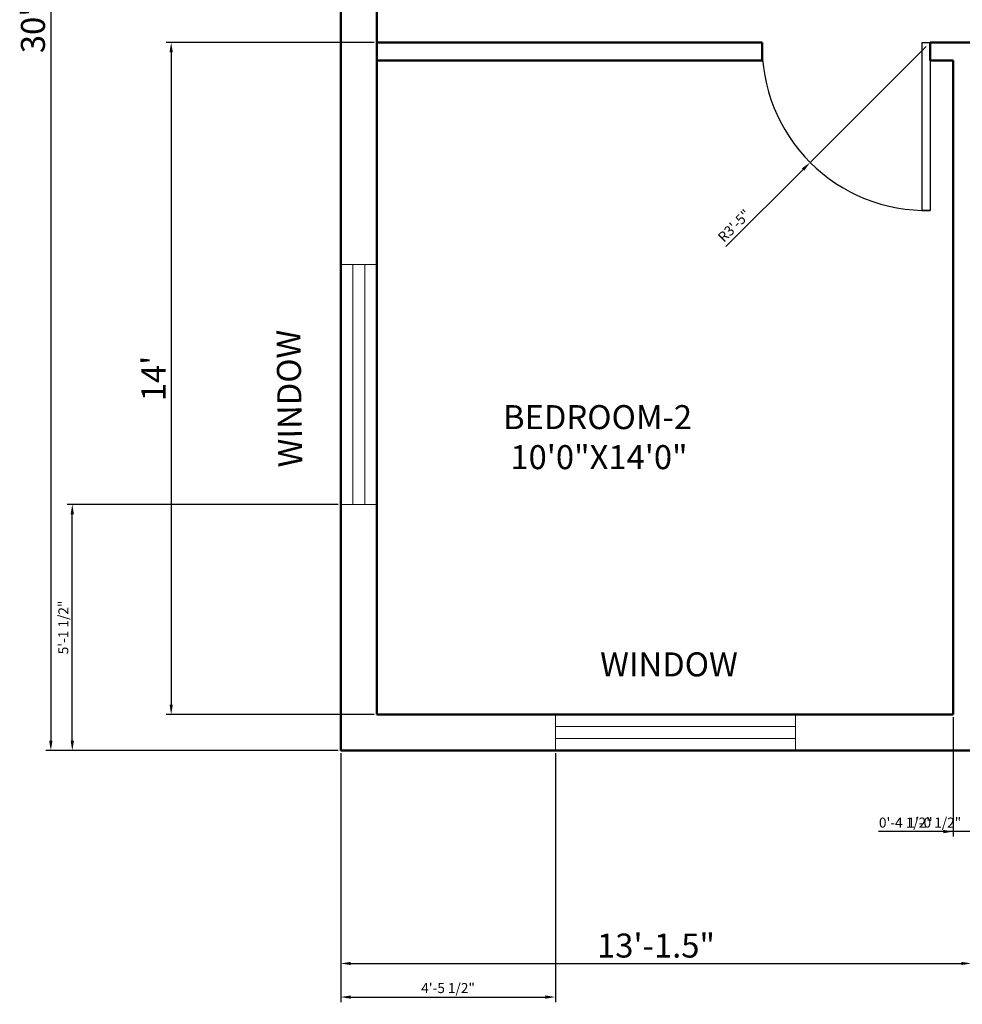
# Model space of a CAD drawing. Units: inches. Extents: x 259417 to 260009, y 246275 to 246915.
# Tile 1 of 4: x 259417 to 259653, y 246340 to 246587. Entities that reach past the tile are written whole.
import ezdxf

# ---------------------------------------------------------------- set-up
doc = ezdxf.new("R2010")
doc.units = ezdxf.units.IN
for name, color, linetype, lineweight in [('A-ANNO-DIMS', 2, 'Continuous', 18), ('A-ANNO-TEXT', 7, 'Continuous', 18), ('A-AREA-IDEN', 7, 'Continuous', 25), ('A-DOOR', 3, 'Continuous', 25), ('A-GLAZ', 4, 'Continuous', 18), ('A-WALL', 7, 'Continuous', 50)]:
    doc.layers.add(name, color=color, linetype=linetype, lineweight=lineweight)
doc.styles.get("Standard").update_dxf_attribs({"font": 'arial.ttf'})
doc.dimstyles.new('ISO-25', dxfattribs={"dimtxt": 2.5, "dimasz": 2.5, "dimexe": 1.25, "dimexo": 0.625, "dimtad": 1, "dimdec": 1, "dimlunit": 3, "dimtxsty": 'Standard', "dimcen": 2.5, "dimadec": 0, "dimazin": 0, "dimtfac": 1, "dimtdec": 1, "dimtmove": 0, "dimatfit": 3, "dimfxl": 1, "dimarcsym": 0})

# ---------------------------------------------------------------- blocks, each defined once
blk = doc.blocks.new('*D9')
at = {"layer": 'A-ANNO-DIMS', "color": 0, "lineweight": -2, "transparency": 16777216}
for p, q in [((259496.97, 246763.84), (259423.92, 246763.84)), ((259425.17, 246761.34), (259425.17, 246406.34)), ((259496.97, 246403.84), (259423.92, 246403.84))]:
    blk.add_line(p, q, dxfattribs=at)
at = {"layer": 'A-ANNO-DIMS', "color": 0, "transparency": 16777216}
for points in [[(259424.75, 246761.34), (259425.59, 246761.34), (259425.17, 246763.84)], [(259424.75, 246406.34), (259425.59, 246406.34), (259425.17, 246403.84)]]:
    blk.add_solid(points, dxfattribs=at)
at = {"layer": 'Defpoints', "color": 0, "transparency": 16777216}
for p in [(259497.59, 246763.84), (259425.17, 246403.84), (259497.59, 246403.84)]:
    blk.add_point(p, dxfattribs=at)
at = {"layer": 'A-ANNO-DIMS', "color": 0, "transparency": 16777216, "insert": (259421.48, 246583.84), "char_height": 6, "attachment_point": 5, "rotation": 90}
blk.add_mtext("30'", dxfattribs=at)
blk = doc.blocks.new('*D10')
at = {"layer": 'A-ANNO-DIMS', "color": 0, "lineweight": -2, "transparency": 16777216}
for p, q in [((259505.97, 246580.84), (259453.98, 246580.84)), ((259455.23, 246578.34), (259455.23, 246415.34)), ((259505.97, 246412.84), (259453.98, 246412.84))]:
    blk.add_line(p, q, dxfattribs=at)
at = {"layer": 'A-ANNO-DIMS', "color": 0, "transparency": 16777216}
for points in [[(259454.81, 246578.34), (259455.64, 246578.34), (259455.23, 246580.84)], [(259454.81, 246415.34), (259455.64, 246415.34), (259455.23, 246412.84)]]:
    blk.add_solid(points, dxfattribs=at)
at = {"layer": 'Defpoints', "color": 0, "transparency": 16777216}
for p in [(259506.59, 246580.84), (259455.23, 246412.84), (259506.59, 246412.84)]:
    blk.add_point(p, dxfattribs=at)
at = {"layer": 'A-ANNO-DIMS', "color": 0, "transparency": 16777216, "insert": (259451.59, 246496.84), "char_height": 6, "attachment_point": 5, "rotation": 90}
blk.add_mtext("14'", dxfattribs=at)
blk = doc.blocks.new('*D20')
at = {"layer": 'A-ANNO-DIMS', "color": 0, "lineweight": -2, "transparency": 16777216}
for p, q in [((259497.59, 246403.22), (259497.59, 246349.38)), ((259655.09, 246403.22), (259655.09, 246349.38)), ((259500.09, 246350.63), (259652.59, 246350.63))]:
    blk.add_line(p, q, dxfattribs=at)
at = {"layer": 'A-ANNO-DIMS', "color": 0, "transparency": 16777216}
for points in [[(259500.09, 246351.04), (259500.09, 246350.21), (259497.59, 246350.63)], [(259652.59, 246351.04), (259652.59, 246350.21), (259655.09, 246350.63)]]:
    blk.add_solid(points, dxfattribs=at)
at = {"layer": 'Defpoints', "color": 0, "transparency": 16777216}
for p in [(259497.59, 246403.84), (259655.09, 246403.84), (259655.09, 246350.63)]:
    blk.add_point(p, dxfattribs=at)
at = {"layer": 'A-ANNO-DIMS', "color": 0, "transparency": 16777216, "insert": (259576.34, 246354.32), "char_height": 6, "attachment_point": 5}
blk.add_mtext('13\'-1.5"', dxfattribs=at)
blk = doc.blocks.new('WIN-60x9')
for p, q in [((0, 9), (0, 0)), ((60, 9), (60, 0)), ((60, 6), (0, 6)), ((60, 3), (0, 3))]:
    blk.add_line(p, q)
blk = doc.blocks.new('*D38')
at = {"layer": 'A-ANNO-DIMS', "color": 0, "lineweight": -2, "transparency": 16777216}
for p, q in [((259496.97, 246465.37), (259429.27, 246465.37)), ((259430.52, 246406.34), (259430.52, 246462.87)), ((259496.97, 246403.84), (259429.27, 246403.84))]:
    blk.add_line(p, q, dxfattribs=at)
at = {"layer": 'A-ANNO-DIMS', "color": 0, "transparency": 16777216}
for points in [[(259430.11, 246462.87), (259430.94, 246462.87), (259430.52, 246465.37)], [(259430.11, 246406.34), (259430.94, 246406.34), (259430.52, 246403.84)]]:
    blk.add_solid(points, dxfattribs=at)
at = {"layer": 'Defpoints', "color": 0, "transparency": 16777216}
for p in [(259430.52, 246465.37), (259497.59, 246465.37), (259497.59, 246403.84)]:
    blk.add_point(p, dxfattribs=at)
at = {"layer": 'A-ANNO-DIMS', "color": 0, "transparency": 16777216, "insert": (259428.61, 246434.61), "char_height": 2.5, "attachment_point": 5, "rotation": 90}
blk.add_mtext('5\'-1 1/2"', dxfattribs=at)
blk = doc.blocks.new('*D39')
at = {"layer": 'A-ANNO-DIMS', "color": 0, "lineweight": -2, "transparency": 16777216}
for p, q in [((259497.59, 246403.22), (259497.59, 246340.98)), ((259551.19, 246403.22), (259551.19, 246340.98)), ((259500.09, 246342.23), (259548.69, 246342.23))]:
    blk.add_line(p, q, dxfattribs=at)
at = {"layer": 'A-ANNO-DIMS', "color": 0, "transparency": 16777216}
for points in [[(259500.09, 246342.64), (259500.09, 246341.81), (259497.59, 246342.23)], [(259548.69, 246342.64), (259548.69, 246341.81), (259551.19, 246342.23)]]:
    blk.add_solid(points, dxfattribs=at)
at = {"layer": 'Defpoints', "color": 0, "transparency": 16777216}
for p in [(259497.59, 246403.84), (259551.19, 246403.84), (259551.19, 246342.23)]:
    blk.add_point(p, dxfattribs=at)
at = {"layer": 'A-ANNO-DIMS', "color": 0, "transparency": 16777216, "insert": (259524.39, 246344.15), "char_height": 2.5, "attachment_point": 5}
blk.add_mtext('4\'-5 1/2"', dxfattribs=at)
blk = doc.blocks.new('*D43')
at = {"layer": 'A-ANNO-DIMS', "color": 0, "lineweight": -2, "transparency": 16777216}
for p, q in [((259650.59, 246412.22), (259650.59, 246382.34)), ((259655.09, 246412.22), (259655.09, 246382.34)), ((259648.09, 246383.59), (259631.87, 246383.59)), ((259655.09, 246383.59), (259650.59, 246383.59)), ((259657.59, 246383.59), (259660.09, 246383.59))]:
    blk.add_line(p, q, dxfattribs=at)
at = {"layer": 'A-ANNO-DIMS', "color": 0, "transparency": 16777216}
for points in [[(259648.09, 246384.01), (259648.09, 246383.17), (259650.59, 246383.59)], [(259657.59, 246384.01), (259657.59, 246383.17), (259655.09, 246383.59)]]:
    blk.add_solid(points, dxfattribs=at)
at = {"layer": 'Defpoints', "color": 0, "transparency": 16777216}
for p in [(259650.59, 246412.84), (259655.09, 246412.84), (259650.59, 246383.59)]:
    blk.add_point(p, dxfattribs=at)
at = {"layer": 'A-ANNO-DIMS', "color": 0, "transparency": 16777216, "insert": (259638.73, 246385.51), "char_height": 2.5, "attachment_point": 5}
blk.add_mtext('0\'-4 1/2"', dxfattribs=at)
blk = doc.blocks.new('*D44')
at = {"layer": 'A-ANNO-DIMS', "color": 0, "lineweight": -2, "transparency": 16777216}
for p, q in [((259655.09, 246412.22), (259655.09, 246382.34)), ((259667.57, 246412.22), (259667.57, 246382.34)), ((259655.09, 246383.59), (259639.11, 246383.59)), ((259665.07, 246383.59), (259657.59, 246383.59))]:
    blk.add_line(p, q, dxfattribs=at)
at = {"layer": 'A-ANNO-DIMS', "color": 0, "transparency": 16777216}
for points in [[(259657.59, 246384.01), (259657.59, 246383.17), (259655.09, 246383.59)], [(259665.07, 246384.01), (259665.07, 246383.17), (259667.57, 246383.59)]]:
    blk.add_solid(points, dxfattribs=at)
at = {"layer": 'Defpoints', "color": 0, "transparency": 16777216}
for p in [(259655.09, 246412.84), (259667.57, 246412.84), (259655.09, 246383.59)]:
    blk.add_point(p, dxfattribs=at)
at = {"layer": 'A-ANNO-DIMS', "color": 0, "transparency": 16777216, "insert": (259645.85, 246385.51), "char_height": 2.5, "attachment_point": 5}
blk.add_mtext('1\'-0 1/2"', dxfattribs=at)
blk = doc.blocks.new('*D67')
at = {"layer": 'A-ANNO-DIMS', "color": 0, "lineweight": -2, "transparency": 16777216}
for p, q in [((259643.83, 246579.84), (259614.83, 246550.84)), ((259593.79, 246529.8), (259613.06, 246549.07))]:
    blk.add_line(p, q, dxfattribs=at)
at = {"layer": 'A-ANNO-DIMS', "color": 0, "transparency": 16777216}
blk.add_solid([(259612.77, 246549.37), (259613.36, 246548.78), (259614.83, 246550.84)], dxfattribs=at)
at = {"layer": 'Defpoints', "color": 0, "transparency": 16777216}
for p in [(259643.83, 246579.84), (259614.83, 246550.84)]:
    blk.add_point(p, dxfattribs=at)
at = {"layer": 'A-ANNO-DIMS', "color": 0, "transparency": 16777216, "insert": (259596.08, 246534.79), "char_height": 2.5, "attachment_point": 5, "rotation": 44.9995}
blk.add_mtext('R3\'-5"', dxfattribs=at)

msp = doc.modelspace()

# ---------------------------------------------------------------- linework, layer by layer
at = {"layer": 'A-DOOR'}
for p, q in [((259642.83, 246538.84), (259642.83, 246580.84)), ((259642.83, 246580.84), (259644.83, 246580.84)), ((259644.83, 246580.84), (259644.83, 246538.84)), ((259644.83, 246538.84), (259642.83, 246538.84))]:
    msp.add_line(p, q, dxfattribs=at)
msp.add_arc((259643.83, 246579.84), 41.01, 178.6028, 271.3972, dxfattribs=at)
at = {"layer": 'A-WALL'}
for p, q in [((259497.59, 246403.84), (259497.59, 246763.84)), ((259506.59, 246412.84), (259506.59, 246754.84)), ((259602.83, 246580.84), (259506.59, 246580.84)), ((259602.83, 246580.84), (259602.83, 246576.34)), ((259644.83, 246580.84), (259644.83, 246576.34)), ((259665.84, 246580.84), (259644.83, 246580.84)), ((259602.83, 246576.34), (259506.59, 246576.34)), ((259650.59, 246576.34), (259644.83, 246576.34)), ((259650.59, 246412.84), (259650.59, 246576.34)), ((259650.59, 246412.84), (259506.59, 246412.84)), ((259667.57, 246403.84), (259497.59, 246403.84))]:
    msp.add_line(p, q, dxfattribs=at)

# ---------------------------------------------------------------- block references
at = {"layer": 'A-GLAZ', "rotation": 269.9999999998505}
msp.add_blockref('WIN-60x9', (259497.59, 246525.37), dxfattribs=at)
at = {"layer": 'A-GLAZ'}
msp.add_blockref('WIN-60x9', (259551.19, 246403.84), dxfattribs=at)

# ---------------------------------------------------------------- texts
at = {"layer": 'A-ANNO-TEXT', "insert": (259482.12, 246465.43), "char_height": 6, "attachment_point": 1, "rotation": 90.8169}
msp.add_mtext_dynamic_manual_height_columns('     WINDOW', width=60.426, gutter_width=12.5, heights=[18.16], dxfattribs=at)
at = {"layer": 'A-ANNO-TEXT', "insert": (259553.21, 246428.38), "char_height": 6, "attachment_point": 1}
msp.add_mtext_dynamic_manual_height_columns('     WINDOW', width=60.426, gutter_width=12.5, heights=[18.16], dxfattribs=at)
at = {"layer": 'A-AREA-IDEN', "insert": (259532.63, 246490.18), "char_height": 6, "attachment_point": 1}
msp.add_mtext_dynamic_manual_height_columns('   BEDROOM-2\\P    10\'0"X14\'0"', width=80.2972, gutter_width=12.5, heights=[23.94], dxfattribs=at)

# ---------------------------------------------------------------- dimensions: what is measured, and where the dimension line sits
at = {"layer": 'A-ANNO-DIMS'}
for base, p1, p2, angle, override, picture, middle in [((259425.17, 246403.84), (259497.59, 246763.84), (259497.59, 246403.84), 90, {"dimtxt": 6, "dimclrd": 0, "dimclre": 0, "dimclrt": 0}, '*D9', (259421.48, 246583.84)), ((259455.23, 246412.84), (259506.59, 246580.84), (259506.59, 246412.84), 90, {"dimtxt": 6, "dimclrd": 0, "dimclre": 0, "dimclrt": 0}, '*D10', (259451.59, 246496.84)), ((259430.52, 246465.37), (259497.59, 246403.84), (259497.59, 246465.37), 90, {"dimdec": 1, "dimlfac": 1, "dimrnd": 0, "dimzin": 1, "dimdsep": 46, "dimlunit": 4, "dimfrac": 2}, '*D38', (259428.61, 246434.61)), ((259650.59, 246383.59), (259655.09, 246412.84), (259650.59, 246412.84), 180, {"dimdec": 1, "dimlfac": 1, "dimrnd": 0, "dimzin": 1, "dimdsep": 46, "dimlunit": 4, "dimfrac": 2}, '*D43', (259638.73, 246385.51)), ((259655.09, 246383.59), (259667.57, 246412.84), (259655.09, 246412.84), 180, {"dimdec": 1, "dimlfac": 1, "dimrnd": 0, "dimzin": 1, "dimdsep": 46, "dimlunit": 4, "dimfrac": 2}, '*D44', (259645.85, 246385.51))]:
    dim = msp.add_linear_dim(base=base, p1=p1, p2=p2, angle=angle, dimstyle='ISO-25', override=override, dxfattribs=at)
    dim.commit()
    dim.dimension.update_dxf_attribs({"geometry": picture, "text_midpoint": middle})
dim = msp.add_radius_dim(center=(259643.83, 246579.84), mpoint=(259614.83, 246550.84), dimstyle='ISO-25', override={"dimdec": 1, "dimlfac": 1, "dimrnd": 0, "dimzin": 1, "dimdsep": 46, "dimlunit": 4, "dimfrac": 2}, dxfattribs=at)
dim.commit()
dim.dimension.update_dxf_attribs({"geometry": '*D67', "text_midpoint": (259597.43, 246533.44), "dimtype": 164})
for base, p2, override, picture, middle in [((259655.09, 246350.63), (259655.09, 246403.84), {"dimtxt": 6, "dimclrd": 0, "dimclre": 0, "dimclrt": 0}, '*D20', (259576.34, 246354.32)), ((259551.19, 246342.23), (259551.19, 246403.84), {"dimdec": 1, "dimlfac": 1, "dimrnd": 0, "dimzin": 1, "dimdsep": 46, "dimlunit": 4, "dimfrac": 2}, '*D39', (259524.39, 246344.15))]:
    dim = msp.add_linear_dim(base=base, p1=(259497.59, 246403.84), p2=p2, dimstyle='ISO-25', override=override, dxfattribs=at)
    dim.commit()
    dim.dimension.update_dxf_attribs({"geometry": picture, "text_midpoint": middle})

doc.saveas('drawing.dxf')
